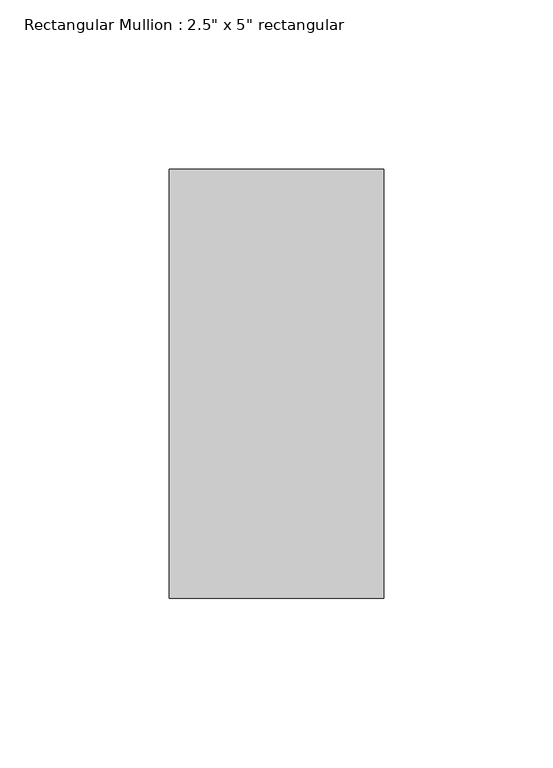
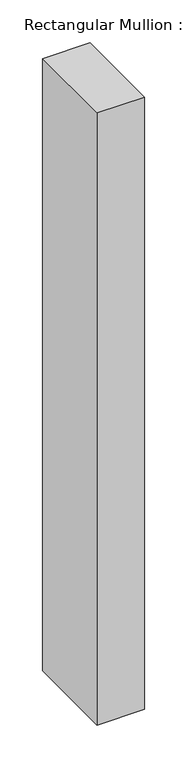
"""IFC4 building model written with IfcOpenShell, lengths in millimetres: member geometry."""

from ifc_helpers import new_model, si_unit, frame, origin, place, context, project, spatial, polyline, outline, extrude, source, transform, mapped, element, save


def member_0adfe7f4(model_context):
    return source(origin(), model_context, "Body", "SweptSolid", [
        extrude(outline(polyline([(0.0, 63.5), (0.0, -63.5), (-63.5, -63.5), (-63.5, 63.5), (0.0, 63.5)])), frame((0.0, 0.0, -871.2851947), z_axis=(0.0, 0.0, 1.0), x_axis=(1.0, 0.0, 0.0)), (0.0, 0.0, 1.0), 871.2851947),
    ])


if __name__ == "__main__":
    model = new_model("IFC4")
    model_context = context("Model", 3, world=origin())
    ifc_project = project(units=[si_unit("LENGTHUNIT", "METRE", prefix="MILLI")], contexts=[model_context])
    site = spatial("IfcSite", under=ifc_project)
    building = spatial("IfcBuilding", under=site)
    placement = place(None, origin())
    member_shape = member_0adfe7f4(model_context)
    element("IfcMember", 1, ObjectType="Rectangular Mullion : 2.5\" x 5\" rectangular", at=placement, inside=building, context=model_context, shape_type="MappedRepresentation", body=[
        mapped(member_shape, transform((0.0, 0.0, 0.0), x_axis=(1.0, 0.0, 0.0), y_axis=(0.0, 1.0, 0.0), z_axis=(0.0, 0.0, 1.0))),
    ])
    save(model, "model.ifc")

# Revit data of these elements
# Type "Rectangular Mullion : 2.5\" x 5\" rectangular"
#   built-in parameter 1007304 = 0.416667 (stored number, unit not read)
#   built-in parameter 1007301 = 0.104167 (stored number, unit not read)
#   built-in parameter 1007300 = 0.104167 (stored number, unit not read)
# Element 1 (IfcMember, "Rectangular Mullion : 2.5\" x 5\" rectangular")
#   Materials on its faces: "Aluminum"
# Materials
#   "Aluminum": class "Metal", colour RGB 247 247 247, transparency 0, Description = "Aluminum 6061", Cost = 0
